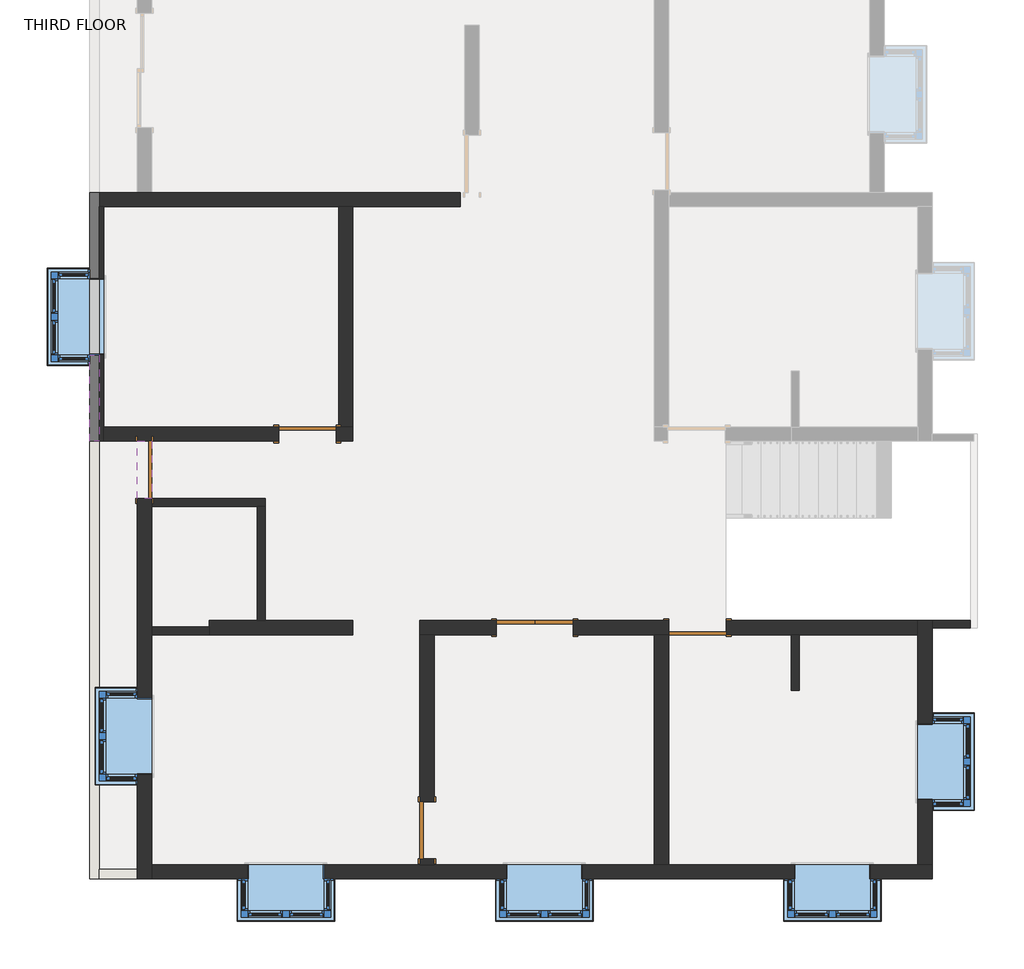
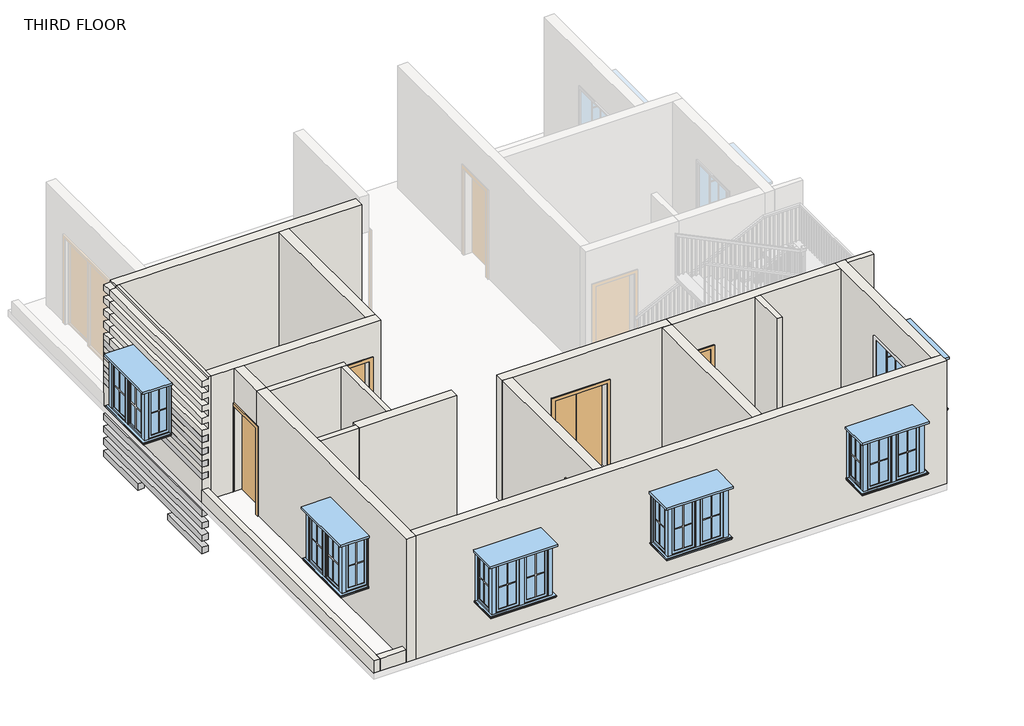
# One storey, part 1 of 4: 20 walls, 8 proxies, 6 windows, 5 doors.
"""IFC4 building model written with IfcOpenShell, lengths in millimetres."""

from ifc_helpers import new_model, si_unit, frame, origin, place, context, project, spatial, polyline, outline, extrude, faceted_brep, transform, mapped, element, save
from components import door_double_flush_panel_4_x7_7c704b5a, door_a90ba1ad, door_0ca8825f, window_bay_casement_box_90_degree_angle_4_x4_x2_07b705a1

model = new_model("IFC4")

# Units and contexts
model_context = context("Model", 3, world=origin())
ifc_project = project(units=[si_unit("LENGTHUNIT", "METRE", prefix="MILLI")], contexts=[model_context])

# Site, building, storey
site = spatial("IfcSite", under=ifc_project)
building = spatial("IfcBuilding", under=site)
storey = spatial("IfcBuildingStorey", under=building, Name="THIRD FLOOR", Elevation=9601.2)

# Proxies
placement = place(None, origin())
element("IfcBuildingElementProxy", 1, Name="Reveal", ObjectType="Reveal", at=placement, inside=storey, context=model_context, shape_type="SweptSolid", body=[
    extrude(outline(polyline([(-7008.3415084, 1592.333346), (-6855.9415084, 1592.333346), (-6855.9415084, 220.733346), (-7008.3415084, 220.733346), (-7008.3415084, 1592.333346)])), frame((0.0, 0.0, 8331.2), z_axis=(0.0, 0.0, 1.0), x_axis=(1.0, 0.0, 0.0)), (0.0, 0.0, 1.0), 152.4),
    extrude(outline(polyline([(-7008.3415084, 4183.133346), (-6855.9415084, 4183.133346), (-6855.9415084, 2811.533346), (-7008.3415084, 2811.533346), (-7008.3415084, 4183.133346)])), frame((0.0, 0.0, 8331.2), z_axis=(0.0, 0.0, 1.0), x_axis=(1.0, 0.0, 0.0)), (0.0, 0.0, 1.0), 152.4),
])
element("IfcBuildingElementProxy", 2, Name="Reveal", ObjectType="Reveal", at=placement, inside=storey, context=model_context, shape_type="SweptSolid", body=[
    extrude(outline(polyline([(-7008.3415084, 4183.133346), (-6855.9415084, 4183.133346), (-6855.9415084, 220.733346), (-7008.3415084, 220.733346), (-7008.3415084, 4183.133346)])), frame((0.0, 0.0, 8636.0), z_axis=(0.0, 0.0, 1.0), x_axis=(1.0, 0.0, 0.0)), (0.0, 0.0, 1.0), 152.4),
])
element("IfcBuildingElementProxy", 3, Name="Reveal", ObjectType="Reveal", at=placement, inside=storey, context=model_context, shape_type="SweptSolid", body=[
    extrude(outline(polyline([(-7008.3415084, 4183.133346), (-6855.9415084, 4183.133346), (-6855.9415084, 220.733346), (-7008.3415084, 220.733346), (-7008.3415084, 4183.133346)])), frame((0.0, 0.0, 8940.8), z_axis=(0.0, 0.0, 1.0), x_axis=(1.0, 0.0, 0.0)), (0.0, 0.0, 1.0), 152.4),
])
element("IfcBuildingElementProxy", 4, Name="Reveal", ObjectType="Reveal", at=placement, inside=storey, context=model_context, shape_type="SweptSolid", body=[
    extrude(outline(polyline([(-7008.3415084, 4183.133346), (-6855.9415084, 4183.133346), (-6855.9415084, 220.733346), (-7008.3415084, 220.733346), (-7008.3415084, 4183.133346)])), frame((0.0, 0.0, 9245.6), z_axis=(0.0, 0.0, 1.0), x_axis=(1.0, 0.0, 0.0)), (0.0, 0.0, 1.0), 152.4),
])
element("IfcBuildingElementProxy", 5, Name="Reveal", ObjectType="Reveal", at=placement, inside=storey, context=model_context, shape_type="SweptSolid", body=[
    extrude(outline(polyline([(-7008.3415084, 4183.133346), (-6855.9415084, 4183.133346), (-6855.9415084, 220.733346), (-7008.3415084, 220.733346), (-7008.3415084, 4183.133346)])), frame((0.0, 0.0, 10160.0), z_axis=(0.0, 0.0, 1.0), x_axis=(1.0, 0.0, 0.0)), (0.0, 0.0, 1.0), 152.4),
])
element("IfcBuildingElementProxy", 6, Name="Reveal", ObjectType="Reveal", at=placement, inside=storey, context=model_context, shape_type="SweptSolid", body=[
    extrude(outline(polyline([(-7008.3415084, 4183.133346), (-6855.9415084, 4183.133346), (-6855.9415084, 220.733346), (-7008.3415084, 220.733346), (-7008.3415084, 4183.133346)])), frame((0.0, 0.0, 10464.8), z_axis=(0.0, 0.0, 1.0), x_axis=(1.0, 0.0, 0.0)), (0.0, 0.0, 1.0), 152.4),
])
element("IfcBuildingElementProxy", 7, Name="Reveal", ObjectType="Reveal", at=placement, inside=storey, context=model_context, shape_type="SweptSolid", body=[
    extrude(outline(polyline([(-7008.3415084, 1592.333346), (-6855.9415084, 1592.333346), (-6855.9415084, 220.733346), (-7008.3415084, 220.733346), (-7008.3415084, 1592.333346)])), frame((0.0, 0.0, 10769.6), z_axis=(0.0, 0.0, 1.0), x_axis=(1.0, 0.0, 0.0)), (0.0, 0.0, 1.0), 152.4),
    extrude(outline(polyline([(-7008.3415084, 4183.133346), (-6855.9415084, 4183.133346), (-6855.9415084, 2811.533346), (-7008.3415084, 2811.533346), (-7008.3415084, 4183.133346)])), frame((0.0, 0.0, 10769.6), z_axis=(0.0, 0.0, 1.0), x_axis=(1.0, 0.0, 0.0)), (0.0, 0.0, 1.0), 152.4),
])
element("IfcBuildingElementProxy", 8, Name="Reveal", ObjectType="Reveal", at=placement, inside=storey, context=model_context, shape_type="SweptSolid", body=[
    extrude(outline(polyline([(-7008.3415084, 1592.333346), (-6855.9415084, 1592.333346), (-6855.9415084, 220.733346), (-7008.3415084, 220.733346), (-7008.3415084, 1592.333346)])), frame((0.0, 0.0, 11074.4), z_axis=(0.0, 0.0, 1.0), x_axis=(1.0, 0.0, 0.0)), (0.0, 0.0, 1.0), 152.4),
    extrude(outline(polyline([(-7008.3415084, 4183.133346), (-6855.9415084, 4183.133346), (-6855.9415084, 2811.533346), (-7008.3415084, 2811.533346), (-7008.3415084, 4183.133346)])), frame((0.0, 0.0, 11074.4), z_axis=(0.0, 0.0, 1.0), x_axis=(1.0, 0.0, 0.0)), (0.0, 0.0, 1.0), 152.4),
])

# Doors
door_double_flush_panel_4_x7_shape = door_double_flush_panel_4_x7_7c704b5a(model_context)
element("IfcDoor", 9, ObjectType="Door-Double-Flush_Panel : 4'x7'", at=placement, inside=storey, context=model_context, shape_type="MappedRepresentation", body=[
    mapped(door_double_flush_panel_4_x7_shape, transform((78.2584916, -2751.066654, 9601.2), x_axis=(1.0, 0.0, 0.0), y_axis=(0.0, 1.0, 0.0), z_axis=(0.0, 0.0, 1.0))),
])
door_shape = door_a90ba1ad(model_context)
element("IfcDoor", 10, ObjectType="Single-Flush : 36\" x 84\"", at=placement, inside=storey, context=model_context, shape_type="MappedRepresentation", body=[
    mapped(door_shape, transform((-1636.2415084, -5976.866654, 9601.2), x_axis=(0.0, -1.0, 0.0), y_axis=(1.0, 0.0, 0.0), z_axis=(0.0, 0.0, 1.0))),
])
door_2_shape = door_0ca8825f(model_context)
element("IfcDoor", 11, ObjectType="Single-Flush : 36\" x 84\"", at=placement, inside=storey, context=model_context, shape_type="MappedRepresentation", body=[
    mapped(door_2_shape, transform((-3541.2415084, 335.033346, 9601.2), x_axis=(1.0, 0.0, 0.0), y_axis=(0.0, 1.0, 0.0), z_axis=(0.0, 0.0, 1.0))),
])
element("IfcDoor", 12, ObjectType="Single-Flush : 36\" x 84\"", at=placement, inside=storey, context=model_context, shape_type="MappedRepresentation", body=[
    mapped(door_2_shape, transform((2669.0584916, -2751.066654, 9601.2), x_axis=(-1.0, 0.0, 0.0), y_axis=(0.0, -1.0, 0.0), z_axis=(0.0, 0.0, 1.0))),
])
element("IfcDoor", 13, ObjectType="Single-Flush : 36\" x 84\"", at=placement, inside=storey, context=model_context, shape_type="MappedRepresentation", body=[
    mapped(door_2_shape, transform((-6132.0415084, -236.466654, 9601.2), x_axis=(0.0, -1.0, 0.0), y_axis=(1.0, 0.0, 0.0), z_axis=(0.0, 0.0, 1.0))),
])

# Walls
element("IfcWall", 14, ObjectType="4.6\"", at=placement, inside=storey, context=model_context, shape_type="SweptSolid", body=[
    extrude(outline(polyline([(7009.1350459, -2753.606654), (6402.8584916, -2753.606654), (6402.8584916, -2636.766654), (7009.1350459, -2636.766654), (7009.1350459, -2753.606654)])), frame((0.0, 0.0, 9601.2), z_axis=(0.0, 0.0, 1.0), x_axis=(1.0, 0.0, 0.0)), (0.0, 0.0, 1.0), 3048.0),
])
element("IfcWall", 15, ObjectType="5\"", at=placement, inside=storey, context=model_context, shape_type="SweptSolid", body=[
    extrude(outline(polyline([(4159.1868368, -3751.826654), (4159.1868368, -2865.366654), (4286.1868368, -2865.366654), (4286.1868368, -3751.826654), (4159.1868368, -3751.826654)])), frame((0.0, 0.0, 9601.2), z_axis=(0.0, 0.0, 1.0), x_axis=(1.0, 0.0, 0.0)), (0.0, 0.0, 1.0), 3048.0),
])
element("IfcWall", 16, ObjectType="5\"", at=placement, inside=storey, context=model_context, shape_type="Brep", body=[
    faceted_brep([(-6017.7415084, -820.666654, 9601.2), (-4341.3415084, -820.666654, 9601.2), (-4214.3415084, -820.666654, 9601.2), (-4214.3415084, -820.666654, 12649.2), (-4341.3415084, -820.666654, 12649.2), (-6017.7415084, -820.666654, 12649.2), (-6017.7415084, -693.666654, 9601.2), (-6017.7415084, -693.666654, 12649.2), (-4214.3415084, -693.666654, 12649.2), (-4214.3415084, -693.666654, 9601.2)], [[[0, 1, 2, 3, 4, 5]], [[6, 7, 8, 9]], [[2, 1, 0, 6, 9]], [[5, 4, 3, 8, 7]], [[0, 5, 7, 6]], [[3, 2, 9, 8]]]),
])
element("IfcWall", 17, ObjectType="5\"", at=placement, inside=storey, context=model_context, shape_type="SweptSolid", body=[
    extrude(outline(polyline([(-4341.3415084, -2636.766654), (-4341.3415084, -820.666654), (-4214.3415084, -820.666654), (-4214.3415084, -2636.766654), (-4341.3415084, -2636.766654)])), frame((0.0, 0.0, 9601.2), z_axis=(0.0, 0.0, 1.0), x_axis=(1.0, 0.0, 0.0)), (0.0, 0.0, 1.0), 3048.0),
])
element("IfcWall", 18, ObjectType="5\"", at=placement, inside=storey, context=model_context, shape_type="SweptSolid", body=[
    extrude(outline(polyline([(-6017.7415084, -2738.366654), (-5103.3415084, -2738.366654), (-5103.3415084, -2865.366654), (-6017.7415084, -2865.366654), (-6017.7415084, -2738.366654)])), frame((0.0, 0.0, 9601.2), z_axis=(0.0, 0.0, 1.0), x_axis=(1.0, 0.0, 0.0)), (0.0, 0.0, 1.0), 3048.0),
])
element("IfcWall", 19, ObjectType="6\"", at=placement, inside=storey, context=model_context, shape_type="Brep", body=[
    faceted_brep([(-7008.3415084, 220.733346, 9601.2), (-7008.3415084, -6751.566654, 9601.2), (-7008.3415084, -6751.566654, 9906.0), (-7008.3415084, 220.733346, 9906.0), (-6855.9415084, 220.733346, 9601.2), (-6855.9415084, 220.733346, 9906.0), (-6855.9415084, -6599.166654, 9906.0), (-6855.9415084, -6751.566654, 9906.0), (-6855.9415084, -6751.566654, 9601.2), (-6855.9415084, -6599.166654, 9601.2)], [[[0, 1, 2, 3]], [[4, 5, 6, 7, 8, 9]], [[1, 0, 4, 9, 8]], [[3, 2, 7, 6, 5]], [[2, 1, 8, 7]], [[0, 3, 5, 4]]]),
])
element("IfcWall", 20, ObjectType="6\"", at=placement, inside=storey, context=model_context, shape_type="SweptSolid", body=[
    extrude(outline(polyline([(-6246.3415084, -6751.566654), (-6855.9415084, -6751.566654), (-6855.9415084, -6599.166654), (-6246.3415084, -6599.166654), (-6246.3415084, -6751.566654)])), frame((0.0, 0.0, 9601.2), z_axis=(0.0, 0.0, 1.0), x_axis=(1.0, 0.0, 0.0)), (0.0, 0.0, 1.0), 304.8),
])
element("IfcWall", 21, ObjectType="9\"", at=placement, inside=storey, context=model_context, shape_type="Brep", body=[
    faceted_brep([(-1108.4404612, 4183.133346, 9601.2), (-6017.7415084, 4183.133346, 9601.2), (-6246.3415084, 4183.133346, 9601.2), (-6855.9415084, 4183.133346, 9601.2), (-7008.3415084, 4183.133346, 9601.2), (-7008.3415084, 4183.133346, 9906.0), (-7008.3415084, 4183.133346, 10160.0), (-6855.9415084, 4183.133346, 10160.0), (-6855.9415084, 4183.133346, 10312.4), (-7008.3415084, 4183.133346, 10312.4), (-7008.3415084, 4183.133346, 10464.8), (-6855.9415084, 4183.133346, 10464.8), (-6855.9415084, 4183.133346, 10617.2), (-7008.3415084, 4183.133346, 10617.2), (-7008.3415084, 4183.133346, 10769.6), (-6855.9415084, 4183.133346, 10769.6), (-6855.9415084, 4183.133346, 10922.0), (-7008.3415084, 4183.133346, 10922.0), (-7008.3415084, 4183.133346, 11074.4), (-6855.9415084, 4183.133346, 11074.4), (-6855.9415084, 4183.133346, 11226.8), (-7008.3415084, 4183.133346, 11226.8), (-7008.3415084, 4183.133346, 11379.2), (-6855.9415084, 4183.133346, 11379.2), (-6855.9415084, 4183.133346, 11531.6), (-7008.3415084, 4183.133346, 11531.6), (-7008.3415084, 4183.133346, 11684.0), (-6855.9415084, 4183.133346, 11684.0), (-6855.9415084, 4183.133346, 11836.4), (-7008.3415084, 4183.133346, 11836.4), (-7008.3415084, 4183.133346, 11988.8), (-6855.9415084, 4183.133346, 11988.8), (-6855.9415084, 4183.133346, 12141.2), (-7008.3415084, 4183.133346, 12141.2), (-7008.3415084, 4183.133346, 12293.6), (-6855.9415084, 4183.133346, 12293.6), (-6855.9415084, 4183.133346, 12446.0), (-7008.3415084, 4183.133346, 12446.0), (-7008.3415084, 4183.133346, 12598.4), (-6855.9415084, 4183.133346, 12598.4), (-6855.9415084, 4183.133346, 12649.2), (-6246.3415084, 4183.133346, 12649.2), (-6017.7415084, 4183.133346, 12649.2), (-1108.4404612, 4183.133346, 12649.2), (-7008.3415084, 3954.533346, 9601.2), (-6779.7415084, 3954.533346, 9601.2), (-3045.9415084, 3954.533346, 9601.2), (-2817.3415084, 3954.533346, 9601.2), (-1108.4404612, 3954.533346, 9601.2), (-1108.4404612, 3954.533346, 12649.2), (-2817.3415084, 3954.533346, 12649.2), (-3045.9415084, 3954.533346, 12649.2), (-6779.7415084, 3954.533346, 12649.2), (-6855.9415084, 3954.533346, 12649.2), (-6855.9415084, 3954.533346, 12598.4), (-7008.3415084, 3954.533346, 12598.4), (-7008.3415084, 3954.533346, 12446.0), (-6855.9415084, 3954.533346, 12446.0), (-6855.9415084, 3954.533346, 12293.6), (-7008.3415084, 3954.533346, 12293.6), (-7008.3415084, 3954.533346, 12141.2), (-6855.9415084, 3954.533346, 12141.2), (-6855.9415084, 3954.533346, 11988.8), (-7008.3415084, 3954.533346, 11988.8), (-7008.3415084, 3954.533346, 11836.4), (-6855.9415084, 3954.533346, 11836.4), (-6855.9415084, 3954.533346, 11684.0), (-7008.3415084, 3954.533346, 11684.0), (-7008.3415084, 3954.533346, 11531.6), (-6855.9415084, 3954.533346, 11531.6), (-6855.9415084, 3954.533346, 11379.2), (-7008.3415084, 3954.533346, 11379.2), (-7008.3415084, 3954.533346, 11226.8), (-6855.9415084, 3954.533346, 11226.8), (-6855.9415084, 3954.533346, 11074.4), (-7008.3415084, 3954.533346, 11074.4), (-7008.3415084, 3954.533346, 10922.0), (-6855.9415084, 3954.533346, 10922.0), (-6855.9415084, 3954.533346, 10769.6), (-7008.3415084, 3954.533346, 10769.6), (-7008.3415084, 3954.533346, 10617.2), (-6855.9415084, 3954.533346, 10617.2), (-6855.9415084, 3954.533346, 10464.8), (-7008.3415084, 3954.533346, 10464.8), (-7008.3415084, 3954.533346, 10312.4), (-6855.9415084, 3954.533346, 10312.4), (-6855.9415084, 3954.533346, 10160.0), (-7008.3415084, 3954.533346, 10160.0)], [[[0, 1, 2, 3, 4, 5, 6, 7, 8, 9, 10, 11, 12, 13, 14, 15, 16, 17, 18, 19, 20, 21, 22, 23, 24, 25, 26, 27, 28, 29, 30, 31, 32, 33, 34, 35, 36, 37, 38, 39, 40, 41, 42, 43]], [[44, 45, 46, 47, 48, 49, 50, 51, 52, 53, 54, 55, 56, 57, 58, 59, 60, 61, 62, 63, 64, 65, 66, 67, 68, 69, 70, 71, 72, 73, 74, 75, 76, 77, 78, 79, 80, 81, 82, 83, 84, 85, 86, 87]], [[4, 3, 2, 1, 0, 48, 47, 46, 45, 44]], [[49, 43, 42, 41, 40, 53, 52, 51, 50]], [[0, 43, 49, 48]], [[4, 44, 87, 6, 5]], [[55, 38, 37, 56]], [[59, 34, 33, 60]], [[63, 30, 29, 64]], [[67, 26, 25, 68]], [[71, 22, 21, 72]], [[75, 18, 17, 76]], [[79, 14, 13, 80]], [[83, 10, 9, 84]], [[39, 54, 53, 40]], [[54, 39, 38, 55]], [[36, 57, 56, 37]], [[57, 36, 35, 58]], [[58, 35, 34, 59]], [[32, 61, 60, 33]], [[61, 32, 31, 62]], [[62, 31, 30, 63]], [[28, 65, 64, 29]], [[65, 28, 27, 66]], [[66, 27, 26, 67]], [[24, 69, 68, 25]], [[69, 24, 23, 70]], [[70, 23, 22, 71]], [[20, 73, 72, 21]], [[73, 20, 19, 74]], [[74, 19, 18, 75]], [[16, 77, 76, 17]], [[77, 16, 15, 78]], [[78, 15, 14, 79]], [[12, 81, 80, 13]], [[81, 12, 11, 82]], [[82, 11, 10, 83]], [[8, 85, 84, 9]], [[85, 8, 7, 86]], [[86, 7, 6, 87]]]),
])
element("IfcWall", 22, ObjectType="9\"", at=placement, inside=storey, context=model_context, shape_type="Brep", body=[
    faceted_brep([(-7008.3415084, 3954.533346, 9601.2), (-7008.3415084, 220.733346, 9601.2), (-7008.3415084, 220.733346, 9906.0), (-7008.3415084, 220.733346, 10160.0), (-7008.3415084, 3954.533346, 10160.0), (-7008.3415084, 2811.533346, 11785.6), (-7008.3415084, 1592.333346, 11785.6), (-7008.3415084, 1592.333346, 11836.4), (-7008.3415084, 220.733346, 11836.4), (-7008.3415084, 220.733346, 11988.8), (-7008.3415084, 3954.533346, 11988.8), (-7008.3415084, 3954.533346, 11836.4), (-7008.3415084, 2811.533346, 11836.4), (-7008.3415084, 220.733346, 12598.4), (-7008.3415084, 3954.533346, 12598.4), (-7008.3415084, 3954.533346, 12446.0), (-7008.3415084, 220.733346, 12446.0), (-7008.3415084, 220.733346, 12293.6), (-7008.3415084, 3954.533346, 12293.6), (-7008.3415084, 3954.533346, 12141.2), (-7008.3415084, 220.733346, 12141.2), (-7008.3415084, 220.733346, 11684.0), (-7008.3415084, 1592.333346, 11684.0), (-7008.3415084, 1592.333346, 11531.6), (-7008.3415084, 220.733346, 11531.6), (-7008.3415084, 2811.533346, 11684.0), (-7008.3415084, 3954.533346, 11684.0), (-7008.3415084, 3954.533346, 11531.6), (-7008.3415084, 2811.533346, 11531.6), (-7008.3415084, 220.733346, 11379.2), (-7008.3415084, 1592.333346, 11379.2), (-7008.3415084, 1592.333346, 11226.8), (-7008.3415084, 220.733346, 11226.8), (-7008.3415084, 2811.533346, 11379.2), (-7008.3415084, 3954.533346, 11379.2), (-7008.3415084, 3954.533346, 11226.8), (-7008.3415084, 2811.533346, 11226.8), (-7008.3415084, 220.733346, 11074.4), (-7008.3415084, 1592.333346, 11074.4), (-7008.3415084, 1592.333346, 10922.0), (-7008.3415084, 220.733346, 10922.0), (-7008.3415084, 2811.533346, 11074.4), (-7008.3415084, 3954.533346, 11074.4), (-7008.3415084, 3954.533346, 10922.0), (-7008.3415084, 2811.533346, 10922.0), (-7008.3415084, 220.733346, 10769.6), (-7008.3415084, 1592.333346, 10769.6), (-7008.3415084, 1592.333346, 10617.2), (-7008.3415084, 220.733346, 10617.2), (-7008.3415084, 2811.533346, 10769.6), (-7008.3415084, 3954.533346, 10769.6), (-7008.3415084, 3954.533346, 10617.2), (-7008.3415084, 2811.533346, 10617.2), (-7008.3415084, 220.733346, 10464.8), (-7008.3415084, 3954.533346, 10464.8), (-7008.3415084, 3954.533346, 10312.4), (-7008.3415084, 220.733346, 10312.4), (-6779.7415084, 220.733346, 9601.2), (-6779.7415084, 449.333346, 9601.2), (-6779.7415084, 3954.533346, 9601.2), (-6779.7415084, 3954.533346, 12649.2), (-6779.7415084, 449.333346, 12649.2), (-6779.7415084, 220.733346, 12649.2), (-6779.7415084, 2811.533346, 11785.6), (-6779.7415084, 2811.533346, 10515.6), (-6779.7415084, 1592.333346, 10515.6), (-6779.7415084, 1592.333346, 11785.6), (-6855.9415084, 220.733346, 9601.2), (-6855.9415084, 3954.533346, 12649.2), (-6855.9415084, 220.733346, 12649.2), (-6855.9415084, 2811.533346, 11785.6), (-6855.9415084, 2811.533346, 11684.0), (-6855.9415084, 2811.533346, 11531.6), (-6855.9415084, 2811.533346, 11379.2), (-6855.9415084, 2811.533346, 11226.8), (-6855.9415084, 2811.533346, 11074.4), (-6855.9415084, 2811.533346, 10922.0), (-6855.9415084, 2811.533346, 10769.6), (-6855.9415084, 2811.533346, 10617.2), (-6855.9415084, 2811.533346, 10515.6), (-6855.9415084, 1592.333346, 10515.6), (-6855.9415084, 1592.333346, 10617.2), (-6855.9415084, 1592.333346, 10769.6), (-6855.9415084, 1592.333346, 10922.0), (-6855.9415084, 1592.333346, 11074.4), (-6855.9415084, 1592.333346, 11226.8), (-6855.9415084, 1592.333346, 11379.2), (-6855.9415084, 1592.333346, 11531.6), (-6855.9415084, 1592.333346, 11684.0), (-6855.9415084, 1592.333346, 11785.6), (-6855.9415084, 220.733346, 12598.4), (-6855.9415084, 220.733346, 12446.0), (-6855.9415084, 220.733346, 12293.6), (-6855.9415084, 220.733346, 12141.2), (-6855.9415084, 220.733346, 11988.8), (-6855.9415084, 220.733346, 11836.4), (-6855.9415084, 220.733346, 11684.0), (-6855.9415084, 220.733346, 11531.6), (-6855.9415084, 220.733346, 11379.2), (-6855.9415084, 220.733346, 11226.8), (-6855.9415084, 220.733346, 11074.4), (-6855.9415084, 220.733346, 10922.0), (-6855.9415084, 220.733346, 10769.6), (-6855.9415084, 220.733346, 10617.2), (-6855.9415084, 220.733346, 10464.8), (-6855.9415084, 220.733346, 10312.4), (-6855.9415084, 220.733346, 10160.0), (-6855.9415084, 3954.533346, 10160.0), (-6855.9415084, 3954.533346, 10312.4), (-6855.9415084, 3954.533346, 10464.8), (-6855.9415084, 3954.533346, 10617.2), (-6855.9415084, 3954.533346, 10769.6), (-6855.9415084, 3954.533346, 10922.0), (-6855.9415084, 3954.533346, 11074.4), (-6855.9415084, 3954.533346, 11226.8), (-6855.9415084, 3954.533346, 11379.2), (-6855.9415084, 3954.533346, 11531.6), (-6855.9415084, 3954.533346, 11684.0), (-6855.9415084, 3954.533346, 11836.4), (-6855.9415084, 3954.533346, 11988.8), (-6855.9415084, 3954.533346, 12141.2), (-6855.9415084, 3954.533346, 12293.6), (-6855.9415084, 3954.533346, 12446.0), (-6855.9415084, 3954.533346, 12598.4), (-6855.9415084, 1592.333346, 11836.4), (-6855.9415084, 2811.533346, 11836.4)], [[[0, 1, 2, 3, 4]], [[5, 6, 7, 8, 9, 10, 11, 12]], [[13, 14, 15, 16]], [[17, 18, 19, 20]], [[21, 22, 23, 24]], [[25, 26, 27, 28]], [[29, 30, 31, 32]], [[33, 34, 35, 36]], [[37, 38, 39, 40]], [[41, 42, 43, 44]], [[45, 46, 47, 48]], [[49, 50, 51, 52]], [[53, 54, 55, 56]], [[57, 58, 59, 60, 61, 62], [63, 64, 65, 66]], [[1, 0, 59, 58, 57, 67]], [[62, 61, 60, 68, 69]], [[64, 63, 70, 71, 25, 28, 72, 73, 33, 36, 74, 75, 41, 44, 76, 77, 49, 52, 78, 79]], [[65, 64, 79, 80]], [[66, 65, 80, 81, 47, 46, 82, 83, 39, 38, 84, 85, 31, 30, 86, 87, 23, 22, 88, 89]], [[63, 66, 89, 6, 5, 70]], [[1, 67, 57, 62, 69, 90, 13, 16, 91, 92, 17, 20, 93, 94, 9, 8, 95, 96, 21, 24, 97, 98, 29, 32, 99, 100, 37, 40, 101, 102, 45, 48, 103, 104, 53, 56, 105, 106, 3, 2]], [[59, 0, 4, 107, 108, 55, 54, 109, 110, 51, 50, 111, 112, 43, 42, 113, 114, 35, 34, 115, 116, 27, 26, 117, 118, 11, 10, 119, 120, 19, 18, 121, 122, 15, 14, 123, 68, 60]], [[123, 90, 69, 68]], [[90, 123, 14, 13]], [[122, 91, 16, 15]], [[91, 122, 121, 92]], [[92, 121, 18, 17]], [[120, 93, 20, 19]], [[93, 120, 119, 94]], [[94, 119, 10, 9]], [[124, 7, 6, 89]], [[7, 124, 95, 8]], [[95, 124, 89, 88, 96]], [[96, 88, 22, 21]], [[12, 125, 70, 5]], [[125, 12, 11, 118]], [[70, 125, 118, 117, 71]], [[71, 117, 26, 25]], [[87, 97, 24, 23]], [[97, 87, 86, 98]], [[98, 86, 30, 29]], [[116, 72, 28, 27]], [[72, 116, 115, 73]], [[73, 115, 34, 33]], [[85, 99, 32, 31]], [[99, 85, 84, 100]], [[100, 84, 38, 37]], [[114, 74, 36, 35]], [[74, 114, 113, 75]], [[75, 113, 42, 41]], [[83, 101, 40, 39]], [[101, 83, 82, 102]], [[102, 82, 46, 45]], [[112, 76, 44, 43]], [[76, 112, 111, 77]], [[77, 111, 50, 49]], [[81, 103, 48, 47]], [[110, 78, 52, 51]], [[103, 81, 80, 79, 78, 110, 109, 104]], [[104, 109, 54, 53]], [[108, 105, 56, 55]], [[105, 108, 107, 106]], [[106, 107, 4, 3]]]),
])
element("IfcWall", 23, ObjectType="9\"", at=placement, inside=storey, context=model_context, shape_type="Brep", body=[
    faceted_brep([(-3084.0415084, 220.733346, 11734.8), (-3084.0415084, 220.733346, 9601.2), (-2817.3415084, 220.733346, 9601.2), (-2817.3415084, 220.733346, 12649.2), (-6017.7415084, 220.733346, 12649.2), (-6246.3415084, 220.733346, 12649.2), (-6779.7415084, 220.733346, 12649.2), (-6779.7415084, 220.733346, 9601.2), (-3998.4415084, 220.733346, 9601.2), (-3998.4415084, 220.733346, 11734.8), (-2817.3415084, 449.333346, 9601.2), (-3045.9415084, 449.333346, 9601.2), (-3084.0415084, 449.333346, 9601.2), (-3084.0415084, 449.333346, 11734.8), (-3998.4415084, 449.333346, 11734.8), (-3998.4415084, 449.333346, 9601.2), (-6779.7415084, 449.333346, 9601.2), (-6779.7415084, 449.333346, 12649.2), (-3045.9415084, 449.333346, 12649.2), (-2817.3415084, 449.333346, 12649.2)], [[[0, 1, 2, 3, 4, 5, 6, 7, 8, 9]], [[10, 11, 12, 13, 14, 15, 16, 17, 18, 19]], [[8, 7, 16, 15]], [[2, 1, 12, 11, 10]], [[6, 5, 4, 3, 19, 18, 17]], [[3, 2, 10, 19]], [[13, 12, 1, 0]], [[14, 13, 0, 9]], [[15, 14, 9, 8]], [[6, 17, 16, 7]]]),
])
element("IfcWall", 24, ObjectType="9\"", at=placement, inside=storey, context=model_context, shape_type="SweptSolid", body=[
    extrude(outline(polyline([(-2817.3415084, 3954.533346), (-2817.3415084, 449.333346), (-3045.9415084, 449.333346), (-3045.9415084, 3954.533346), (-2817.3415084, 3954.533346)])), frame((0.0, 0.0, 9601.2), z_axis=(0.0, 0.0, 1.0), x_axis=(1.0, 0.0, 0.0)), (0.0, 0.0, 1.0), 3048.0),
])
element("IfcWall", 25, ObjectType="9\"", at=placement, inside=storey, context=model_context, shape_type="Brep", body=[
    faceted_brep([(-6246.3415084, -693.666654, 9601.2), (-6246.3415084, -6599.166654, 9601.2), (-6246.3415084, -6751.566654, 9601.2), (-6246.3415084, -6751.566654, 9906.0), (-6246.3415084, -6751.566654, 12649.2), (-6246.3415084, -693.666654, 12649.2), (-6246.3415084, -693.666654, 11734.8), (-6246.3415084, -3868.666654, 11785.6), (-6246.3415084, -5087.866654, 11785.6), (-6246.3415084, -5087.866654, 10515.6), (-6246.3415084, -3868.666654, 10515.6), (-6017.7415084, -693.666654, 9601.2), (-6017.7415084, -693.666654, 11734.8), (-6017.7415084, -693.666654, 12649.2), (-6017.7415084, -820.666654, 12649.2), (-6017.7415084, -2738.366654, 12649.2), (-6017.7415084, -2865.366654, 12649.2), (-6017.7415084, -6522.966654, 12649.2), (-6017.7415084, -6751.566654, 12649.2), (-6017.7415084, -6751.566654, 9601.2), (-6017.7415084, -6522.966654, 9601.2), (-6017.7415084, -2865.366654, 9601.2), (-6017.7415084, -2738.366654, 9601.2), (-6017.7415084, -820.666654, 9601.2), (-6017.7415084, -3868.666654, 11785.6), (-6017.7415084, -3868.666654, 10515.6), (-6017.7415084, -5087.866654, 10515.6), (-6017.7415084, -5087.866654, 11785.6)], [[[0, 1, 2, 3, 4, 5, 6], [7, 8, 9, 10]], [[11, 12, 13, 14, 15, 16, 17, 18, 19, 20, 21, 22, 23], [24, 25, 26, 27]], [[2, 1, 0, 11, 23, 22, 21, 20, 19]], [[5, 4, 18, 17, 16, 15, 14, 13]], [[0, 6, 5, 13, 12, 11]], [[25, 24, 7, 10]], [[26, 25, 10, 9]], [[27, 26, 9, 8]], [[24, 27, 8, 7]], [[2, 19, 18, 4, 3]]]),
])
element("IfcWall", 26, ObjectType="9\"", at=placement, inside=storey, context=model_context, shape_type="Brep", body=[
    faceted_brep([(-2817.3415084, -2636.766654, 9601.2), (-4214.3415084, -2636.766654, 9601.2), (-4341.3415084, -2636.766654, 9601.2), (-5103.3415084, -2636.766654, 9601.2), (-5103.3415084, -2636.766654, 12649.2), (-4341.3415084, -2636.766654, 12649.2), (-4214.3415084, -2636.766654, 12649.2), (-2817.3415084, -2636.766654, 12649.2), (-2817.3415084, -2865.366654, 9601.2), (-2817.3415084, -2865.366654, 12649.2), (-5103.3415084, -2865.366654, 12649.2), (-5103.3415084, -2865.366654, 9601.2), (-5103.3415084, -2738.366654, 9601.2), (-5103.3415084, -2738.366654, 12649.2)], [[[0, 1, 2, 3, 4, 5, 6, 7]], [[8, 9, 10, 11]], [[3, 2, 1, 0, 8, 11, 12]], [[4, 3, 12, 11, 10, 13]], [[7, 6, 5, 4, 13, 10, 9]], [[0, 7, 9, 8]]]),
])
element("IfcWall", 27, ObjectType="9\"", at=placement, inside=storey, context=model_context, shape_type="Brep", body=[
    faceted_brep([(2211.8584916, -2865.366654, 12649.2), (1983.2584916, -2865.366654, 12649.2), (-1521.9415084, -2865.366654, 12649.2), (-1750.5415084, -2865.366654, 12649.2), (-1750.5415084, -2865.366654, 9601.2), (-1521.9415084, -2865.366654, 9601.2), (-531.3415084, -2865.366654, 9601.2), (-531.3415084, -2865.366654, 11734.8), (687.8584916, -2865.366654, 11734.8), (687.8584916, -2865.366654, 9601.2), (1983.2584916, -2865.366654, 9601.2), (2211.8584916, -2865.366654, 9601.2), (2211.8584916, -2865.366654, 11734.8), (-1750.5415084, -2636.766654, 12649.2), (2211.8584916, -2636.766654, 12649.2), (2211.8584916, -2636.766654, 11734.8), (2211.8584916, -2636.766654, 9601.2), (687.8584916, -2636.766654, 9601.2), (687.8584916, -2636.766654, 11734.8), (-531.3415084, -2636.766654, 11734.8), (-531.3415084, -2636.766654, 9601.2), (-1750.5415084, -2636.766654, 9601.2)], [[[0, 1, 2, 3, 4, 5, 6, 7, 8, 9, 10, 11, 12]], [[13, 14, 15, 16, 17, 18, 19, 20, 21]], [[16, 11, 10, 9, 17]], [[4, 21, 20, 6, 5]], [[3, 2, 1, 0, 14, 13]], [[0, 12, 11, 16, 15, 14]], [[4, 3, 13, 21]], [[8, 18, 17, 9]], [[18, 8, 7, 19]], [[19, 7, 6, 20]]]),
])
element("IfcWall", 28, ObjectType="9\"", at=placement, inside=storey, context=model_context, shape_type="SweptSolid", body=[
    extrude(outline(polyline([(1983.2584916, -6522.966654), (1983.2584916, -2865.366654), (2211.8584916, -2865.366654), (2211.8584916, -6522.966654), (1983.2584916, -6522.966654)])), frame((0.0, 0.0, 9601.2), z_axis=(0.0, 0.0, 1.0), x_axis=(1.0, 0.0, 0.0)), (0.0, 0.0, 1.0), 3048.0),
])
element("IfcWall", 29, ObjectType="9\"", at=placement, inside=storey, context=model_context, shape_type="Brep", body=[
    faceted_brep([(-6017.7415084, -6751.566654, 12649.2), (-6017.7415084, -6751.566654, 9601.2), (6402.8584916, -6751.566654, 9601.2), (6402.8584916, -6751.566654, 12649.2), (-378.9415084, -6751.566654, 11785.6), (840.2584916, -6751.566654, 11785.6), (840.2584916, -6751.566654, 10515.6), (-378.9415084, -6751.566654, 10515.6), (4205.7584916, -6751.566654, 11785.6), (5424.9584916, -6751.566654, 11785.6), (5424.9584916, -6751.566654, 10515.6), (4205.7584916, -6751.566654, 10515.6), (-4493.7415084, -6751.566654, 11785.6), (-3274.5415084, -6751.566654, 11785.6), (-3274.5415084, -6751.566654, 10515.6), (-4493.7415084, -6751.566654, 10515.6), (-6017.7415084, -6522.966654, 9601.2), (-6017.7415084, -6522.966654, 12649.2), (-1750.5415084, -6522.966654, 12649.2), (-1521.9415084, -6522.966654, 12649.2), (1983.2584916, -6522.966654, 12649.2), (2211.8584916, -6522.966654, 12649.2), (6174.2584916, -6522.966654, 12649.2), (6402.8584916, -6522.966654, 12649.2), (6402.8584916, -6522.966654, 9601.2), (6174.2584916, -6522.966654, 9601.2), (2211.8584916, -6522.966654, 9601.2), (1983.2584916, -6522.966654, 9601.2), (-1521.9415084, -6522.966654, 9601.2), (-1750.5415084, -6522.966654, 9601.2), (-378.9415084, -6522.966654, 11785.6), (-378.9415084, -6522.966654, 10515.6), (840.2584916, -6522.966654, 10515.6), (840.2584916, -6522.966654, 11785.6), (4205.7584916, -6522.966654, 11785.6), (4205.7584916, -6522.966654, 10515.6), (5424.9584916, -6522.966654, 10515.6), (5424.9584916, -6522.966654, 11785.6), (-4493.7415084, -6522.966654, 11785.6), (-4493.7415084, -6522.966654, 10515.6), (-3274.5415084, -6522.966654, 10515.6), (-3274.5415084, -6522.966654, 11785.6)], [[[0, 1, 2, 3], [4, 5, 6, 7], [8, 9, 10, 11], [12, 13, 14, 15]], [[16, 17, 18, 19, 20, 21, 22, 23, 24, 25, 26, 27, 28, 29], [30, 31, 32, 33], [34, 35, 36, 37], [38, 39, 40, 41]], [[2, 1, 16, 29, 28, 27, 26, 25, 24]], [[0, 3, 23, 22, 21, 20, 19, 18, 17]], [[3, 2, 24, 23]], [[31, 30, 4, 7]], [[32, 31, 7, 6]], [[33, 32, 6, 5]], [[30, 33, 5, 4]], [[35, 34, 8, 11]], [[36, 35, 11, 10]], [[37, 36, 10, 9]], [[34, 37, 9, 8]], [[39, 38, 12, 15]], [[40, 39, 15, 14]], [[41, 40, 14, 13]], [[38, 41, 13, 12]], [[0, 17, 16, 1]]]),
])
element("IfcWall", 30, ObjectType="9\"", at=placement, inside=storey, context=model_context, shape_type="Brep", body=[
    faceted_brep([(6402.8584916, -6522.966654, 9601.2), (6402.8584916, -2753.606654, 9601.2), (6402.8584916, -2636.766654, 9601.2), (6402.8584916, -2636.766654, 12649.2), (6402.8584916, -2753.606654, 12649.2), (6402.8584916, -6522.966654, 12649.2), (6402.8584916, -5494.266654, 11785.6), (6402.8584916, -4275.066654, 11785.6), (6402.8584916, -4275.066654, 10515.6), (6402.8584916, -5494.266654, 10515.6), (6174.2584916, -6522.966654, 9601.2), (6174.2584916, -6522.966654, 12649.2), (6174.2584916, -2865.366654, 12649.2), (6174.2584916, -2636.766654, 12649.2), (6174.2584916, -2636.766654, 9601.2), (6174.2584916, -2865.366654, 9601.2), (6174.2584916, -5494.266654, 11785.6), (6174.2584916, -5494.266654, 10515.6), (6174.2584916, -4275.066654, 10515.6), (6174.2584916, -4275.066654, 11785.6)], [[[0, 1, 2, 3, 4, 5], [6, 7, 8, 9]], [[10, 11, 12, 13, 14, 15], [16, 17, 18, 19]], [[2, 1, 0, 10, 15, 14]], [[5, 4, 3, 13, 12, 11]], [[0, 5, 11, 10]], [[3, 2, 14, 13]], [[17, 16, 6, 9]], [[18, 17, 9, 8]], [[19, 18, 8, 7]], [[16, 19, 7, 6]]]),
])
element("IfcWall", 31, ObjectType="9\"", at=placement, inside=storey, context=model_context, shape_type="Brep", body=[
    faceted_brep([(2211.8584916, -2636.766654, 12649.2), (6174.2584916, -2636.766654, 12649.2), (6174.2584916, -2636.766654, 9601.2), (3126.2584916, -2636.766654, 9601.2), (3126.2584916, -2636.766654, 11734.8), (2211.8584916, -2636.766654, 11734.8), (6174.2584916, -2865.366654, 12649.2), (4286.1868368, -2865.366654, 12649.2), (4159.1868368, -2865.366654, 12649.2), (2211.8584916, -2865.366654, 12649.2), (2211.8584916, -2865.366654, 11734.8), (3126.2584916, -2865.366654, 11734.8), (3126.2584916, -2865.366654, 9601.2), (4159.1868368, -2865.366654, 9601.2), (4286.1868368, -2865.366654, 9601.2), (6174.2584916, -2865.366654, 9601.2)], [[[0, 1, 2, 3, 4, 5]], [[6, 7, 8, 9, 10, 11, 12, 13, 14, 15]], [[2, 15, 14, 13, 12, 3]], [[1, 0, 9, 8, 7, 6]], [[2, 1, 6, 15]], [[9, 0, 5, 10]], [[4, 11, 10, 5]], [[11, 4, 3, 12]]]),
])
element("IfcWall", 32, ObjectType="9\"", at=placement, inside=storey, context=model_context, shape_type="SweptSolid", body=[
    extrude(outline(polyline([(-6434.066654, 11734.8), (-6434.066654, 9601.2), (-6522.966654, 9601.2), (-6522.966654, 12649.2), (-2865.366654, 12649.2), (-2865.366654, 9601.2), (-5519.666654, 9601.2), (-5519.666654, 11734.8), (-6434.066654, 11734.8)])), frame((-1750.5415084, 0.0, 0.0), z_axis=(1.0, 0.0, 0.0), x_axis=(0.0, 1.0, 0.0)), (0.0, 0.0, 1.0), 228.6),
])
element("IfcWall", 33, ObjectType="9\"", at=placement, inside=storey, context=model_context, shape_type="SweptSolid", body=[
    extrude(outline(polyline([(-6017.7415084, 220.733346), (-6017.7415084, -693.666654), (-6246.3415084, -693.666654), (-6246.3415084, 220.733346), (-6017.7415084, 220.733346)])), frame((0.0, 0.0, 11734.8), z_axis=(0.0, 0.0, 1.0), x_axis=(1.0, 0.0, 0.0)), (0.0, 0.0, 1.0), 914.4),
])

# Windows
window_bay_casement_box_90_degree_angle_4_x4_x2_shape = window_bay_casement_box_90_degree_angle_4_x4_x2_07b705a1(model_context)
element("IfcWindow", 34, ObjectType="Window-Bay-Casement-Box-90_Degree_Angle : 4'X4'X2'", at=placement, inside=storey, context=model_context, shape_type="MappedRepresentation", body=[
    mapped(window_bay_casement_box_90_degree_angle_4_x4_x2_shape, transform((-6894.0415084, 2201.933346, 9906.0), x_axis=(0.0, 1.0, 0.0), y_axis=(-1.0, 0.0, 0.0), z_axis=(0.0, 0.0, 1.0))),
])
element("IfcWindow", 35, ObjectType="Window-Bay-Casement-Box-90_Degree_Angle : 4'X4'X2'", at=placement, inside=storey, context=model_context, shape_type="MappedRepresentation", body=[
    mapped(window_bay_casement_box_90_degree_angle_4_x4_x2_shape, transform((-6132.0415084, -4478.266654, 9906.0), x_axis=(0.0, 1.0, 0.0), y_axis=(-1.0, 0.0, 0.0), z_axis=(0.0, 0.0, 1.0))),
])
element("IfcWindow", 36, ObjectType="Window-Bay-Casement-Box-90_Degree_Angle : 4'X4'X2'", at=placement, inside=storey, context=model_context, shape_type="MappedRepresentation", body=[
    mapped(window_bay_casement_box_90_degree_angle_4_x4_x2_shape, transform((6288.5584916, -4884.666654, 9906.0), x_axis=(0.0, -1.0, 0.0), y_axis=(1.0, 0.0, 0.0), z_axis=(0.0, 0.0, 1.0))),
])
element("IfcWindow", 37, ObjectType="Window-Bay-Casement-Box-90_Degree_Angle : 4'X4'X2'", at=placement, inside=storey, context=model_context, shape_type="MappedRepresentation", body=[
    mapped(window_bay_casement_box_90_degree_angle_4_x4_x2_shape, transform((230.6584916, -6637.266654, 9906.0), x_axis=(-1.0, 0.0, 0.0), y_axis=(0.0, -1.0, 0.0), z_axis=(0.0, 0.0, 1.0))),
])
element("IfcWindow", 38, ObjectType="Window-Bay-Casement-Box-90_Degree_Angle : 4'X4'X2'", at=placement, inside=storey, context=model_context, shape_type="MappedRepresentation", body=[
    mapped(window_bay_casement_box_90_degree_angle_4_x4_x2_shape, transform((4815.3584916, -6637.266654, 9906.0), x_axis=(-1.0, 0.0, 0.0), y_axis=(0.0, -1.0, 0.0), z_axis=(0.0, 0.0, 1.0))),
])
element("IfcWindow", 39, ObjectType="Window-Bay-Casement-Box-90_Degree_Angle : 4'X4'X2'", at=placement, inside=storey, context=model_context, shape_type="MappedRepresentation", body=[
    mapped(window_bay_casement_box_90_degree_angle_4_x4_x2_shape, transform((-3884.1415084, -6637.266654, 9906.0), x_axis=(-1.0, 0.0, 0.0), y_axis=(0.0, -1.0, 0.0), z_axis=(0.0, 0.0, 1.0))),
])

save(model, "model.ifc")

# Revit data of these elements
# Type "Door-Double-Flush_Panel : 4'x7'"
#   Type Mark = "9"
#   Construction Type Id = "DOOR"
#   Assembly Code = "C1020"
#   Analytic Construction = "Wooden"
#   Thickness = 0' - 2"
#   Thermal Resistance (R) = 2.5876 (h·ft²·°F)/BTU
#   Swing Angle [instance default] = 90.00°
#   Panel Width = 2' - 0"
#   Heat Transfer Coefficient (U) = 0.3865 BTU/(h·ft²·°F)
#   Height = 7' - 0"
#   Trim Projection Ext = 0' - 1"
#   Trim Projection Int = 0' - 1"
#   Trim Width = 0' - 3"
#   Width = 4' - 0"
#   Define Thermal Properties by = 1
#   Panel Material = Wood - Birch - Solid Stained Light Low Gloss
#   Trim Material = Paint - Sienna
#   Visual Light Transmittance = 0
#   Solar Heat Gain Coefficient = 0
#   Function = (empty or 0)
#   Wall Closure = (empty or 0)
# Type "Single-Flush : 36\" x 84\""
#   Type Mark = "1"
#   Construction Type Id = "MDOOR"
#   Assembly Code = "C1020"
#   Analytic Construction = "Metal"
#   Thickness = 0' - 2"
#   Heat Transfer Coefficient (U) = 0.651978 BTU/(h·ft²·°F)
#   Height = 7' - 0"
#   Trim Projection Ext = 0' - 1"
#   Trim Projection Int = 0' - 1"
#   Trim Width = 0' - 3"
#   Width = 3' - 0"
#   Define Thermal Properties by = 1
#   Define Thermal Properties by = 1
#   Door Material = Door - Panel
#   Frame Material = Door - Frame
#   Visual Light Transmittance = 0
#   Solar Heat Gain Coefficient = 0
#   Function = (empty or 0)
#   Wall Closure = (empty or 0)
# Type "4.6\""
#   Assembly Code = "B2010"
#   Layers, outside or top first: 0' - 4 77/128" no material (function 1)
# Type "5\""
#   Assembly Code = "B2010"
#   Layers, outside or top first: 0' - 5" no material (function 1)
# Type "6\""
#   Assembly Code = "B2010"
#   Layers, outside or top first: 0' - 6" no material (function 1)
# Type "9\""
#   Assembly Code = "B2010"
#   Layers, outside or top first: 0' - 9" "WALL 1" (function 1)
# Type "Window-Bay-Casement-Box-90_Degree_Angle : 4'X4'X2'"
#   Type Mark = "20"
#   Fire Rating = "0.5h"
#   Assembly Code = "B2020100"
#   Analytic Construction = "1/8 in Pilkington single glazing"
#   Width = 4' - 0"
#   Wall Thickness [instance default] = 0' - 6"
#   Visual Light Transmittance = 0.9
#   Trim Width = 4' - 8"
#   Trim Height = 4' - 0"
#   Thermal Resistance (R) = 1.5394 (h·ft²·°F)/BTU
#   Solar Heat Gain Coefficient = 0.86
#   Rough Width = 4' - 0 1/2"
#   Rough Height = 4' - 0 1/2"
#   Height 1 = 4' - 2"
#   Height = 4' - 0"
#   Heat Transfer Coefficient (U) = 0.6496 BTU/(h·ft²·°F)
#   Depth = 2' - 0"
#   Default Sill Height = 2' - 0"
#   Muntin Visibility = yes
#   Interior Trim Visibility [instance default] = yes
#   Exterior Trim Visibility [instance default] = yes
#   Muntin Pattern = Muntin Pattern_2x2 : Muntin Pattern_2x2
#   Interior Trim Material = Wood - Stained
#   Exterior Trim Material = Clad - White
#   Exterior Trim = element 423684
#   Interior Trim = Trim-Window-Interior-Flat : Picture Frame
#   Interior Frame Material = Wood - Stained
#   Glass Panel Material = Glass
#   Exterior Frame Material = Clad - White
#   Wall Closure = (empty or 0)
# Element 9 (IfcDoor, "Door-Double-Flush_Panel : 4'x7'")
#   Swing Angle = 90.00°
#   Phase Created = New Construction
#   Materials on its faces: "Paint - Sienna", "Wood - Birch - Solid Stained Light Low Gloss"
# Elements 10, 11, 12, 13 (IfcDoor, "Single-Flush : 36\" x 84\"")
#   Phase Created = New Construction
#   Materials on its faces: "Door - Frame", "Door - Panel"
# Element 14 (IfcWall, "4.6\"")
#   Top Offset = -0' - 6"
#   Base Offset = 0' - 0"
#   wall height = 10' - 0"
#   Phase Created = New Construction
#   Base Constraint = THIRD FLOOR
#   Top Constraint = FOURTH FLOOR
#   Materials on its faces: "Default Wall", "WALL 1"
# Elements 15, 16, 17, 18 (IfcWall, "5\"")
#   Top Offset = -0' - 6"
#   Base Offset = 0' - 0"
#   wall height = 10' - 0"
#   Phase Created = New Construction
#   Base Constraint = THIRD FLOOR
#   Top Constraint = FOURTH FLOOR
#   Materials on its faces: "Default Wall"
# Element 19 (IfcWall, "6\"")
#   Top Offset = -0' - 6"
#   Base Offset = 0' - 0"
#   Unconnected Height = 1' - 0"
#   wall height = 1' - 0"
#   Phase Created = New Construction
#   Base Constraint = THIRD FLOOR
#   Materials on its faces: "Default Wall", "WALL 4"
# Element 20 (IfcWall, "6\"")
#   Top Offset = -0' - 6"
#   Base Offset = 0' - 0"
#   Unconnected Height = 1' - 0"
#   wall height = 1' - 0"
#   Phase Created = New Construction
#   Base Constraint = THIRD FLOOR
#   Materials on its faces: "Default Wall"
# Elements 21, 22, 29 (IfcWall, "9\"")
#   Top Offset = -0' - 6"
#   Base Offset = 0' - 0"
#   wall height = 10' - 0"
#   Phase Created = New Construction
#   Base Constraint = THIRD FLOOR
#   Top Constraint = FOURTH FLOOR
#   Materials on its faces: "WALL 1", "WALL 2"
# Elements 23, 24, 26, 27, 28, 30, 31, 32, 33 (IfcWall, "9\"")
#   Top Offset = -0' - 6"
#   Base Offset = 0' - 0"
#   wall height = 10' - 0"
#   Phase Created = New Construction
#   Base Constraint = THIRD FLOOR
#   Top Constraint = FOURTH FLOOR
#   Materials on its faces: "WALL 1"
# Element 25 (IfcWall, "9\"")
#   Top Offset = -0' - 6"
#   Base Offset = 0' - 0"
#   wall height = 10' - 0"
#   Phase Created = New Construction
#   Base Constraint = THIRD FLOOR
#   Top Constraint = FOURTH FLOOR
#   Materials on its faces: "WALL 1", "Default Wall", "WALL 2"
# Element 34 (IfcWindow, "Window-Bay-Casement-Box-90_Degree_Angle : 4'X4'X2'")
#   Mark = "40"
#   Phase Created = New Construction
#   Materials on its faces: "Clad - White", "Wood - Stained", "Glass"
# Element 35 (IfcWindow, "Window-Bay-Casement-Box-90_Degree_Angle : 4'X4'X2'")
#   Mark = "41"
#   Phase Created = New Construction
#   Materials on its faces: "Clad - White", "Wood - Stained", "Glass"
# Element 36 (IfcWindow, "Window-Bay-Casement-Box-90_Degree_Angle : 4'X4'X2'")
#   Mark = "42"
#   Phase Created = New Construction
#   Materials on its faces: "Clad - White", "Wood - Stained", "Glass"
# Element 37 (IfcWindow, "Window-Bay-Casement-Box-90_Degree_Angle : 4'X4'X2'")
#   Mark = "47"
#   Phase Created = New Construction
#   Materials on its faces: "Clad - White", "Wood - Stained", "Glass"
# Element 38 (IfcWindow, "Window-Bay-Casement-Box-90_Degree_Angle : 4'X4'X2'")
#   Mark = "48"
#   Phase Created = New Construction
#   Materials on its faces: "Clad - White", "Wood - Stained", "Glass"
# Element 39 (IfcWindow, "Window-Bay-Casement-Box-90_Degree_Angle : 4'X4'X2'")
#   Mark = "49"
#   Phase Created = New Construction
#   Materials on its faces: "Clad - White", "Wood - Stained", "Glass"
# Materials
#   "Wood - Birch - Solid Stained Light Low Gloss": class "Wood", colour RGB 210 159 95, transparency 0, Cost = 0
#   "Paint - Sienna": colour RGB 118 70 51, transparency 0, Cost = 0
#   "Door - Panel": class "Wood", colour RGB 210 159 95, transparency 0, Cost = 0
#   "Door - Frame": colour RGB 118 70 51, transparency 0, Cost = 0
#   "WALL 1": class "Generic", colour RGB 233 224 215, transparency 0, Cost = 0
#   "Wood - Stained": class "Wood", colour RGB 224 178 126, transparency 0, Cost = 0
#   "Clad - White": class "Wood", colour RGB 242 242 238, transparency 0, Cost = 0
#   "Glass": class "Glass", colour RGB 0 128 192, transparency 0.75, Description = "Soda Lime Glass", Cost = 0
#   "Default Wall": colour RGB 128 128 128, transparency 0, Cost = 0
#   "WALL 4": class "Generic", colour RGB 32 32 32, transparency 0, Cost = 0
#   "WALL 2": class "Generic", colour RGB 52 58 64, transparency 0, Cost = 0
